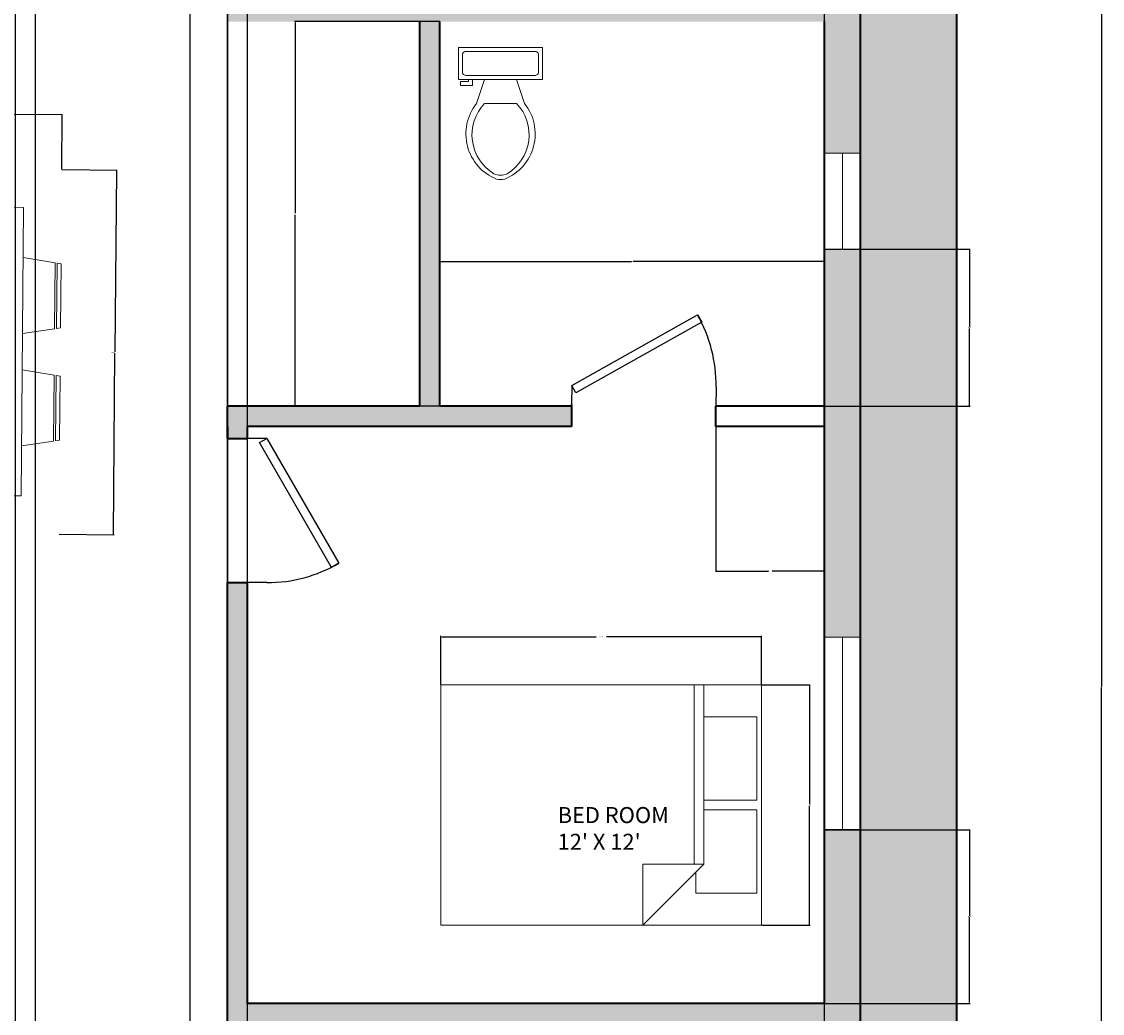
# Model space of a CAD drawing. Units: inches. Extents: x -7 to 546, y -27 to 766.
# Tile 8 of 9: x 276 to 546, y 276 to 524. Entities that reach past the tile are written whole.
import ezdxf

# ---------------------------------------------------------------- set-up
doc = ezdxf.new("R2010")
doc.units = ezdxf.units.IN
doc.header["$MEASUREMENT"] = 0
for name, color, linetype, lineweight in [('A-ANNO-DIMS', 2, 'Continuous', 18), ('A-AREA-IDEN', 7, 'Continuous', 18), ('A-FLOR-FIXT', 9, 'Continuous', 18), ('A-WALL', 7, 'Continuous', 35), ('C-PROP', 7, 'Continuous', 35), ('doors', 40, 'Continuous', 25), ('furniture', 220, 'Continuous', 18), ('window', 30, 'Continuous', 20)]:
    doc.layers.add(name, color=color, linetype=linetype, lineweight=lineweight)
doc.layers.add('A-WALL-PATT', color=251, linetype='Continuous', lineweight=13, true_color=0x636466)
doc.layers.add('L-PLNT-PATT', color=85, linetype='Continuous', lineweight=13, true_color=0x58ba48)
doc.styles.get("Standard").update_dxf_attribs({"font": 'arial.ttf'})
doc.dimstyles.get("Standard").update_dxf_attribs({"dimtxt": 0.18, "dimasz": 0.18, "dimexe": 0.18, "dimexo": 0.0625, "dimgap": 0.09, "dimtad": 0, "dimtih": 1, "dimtoh": 1, "dimdec": 4, "dimzin": 0, "dimdsep": 46, "dimtxsty": 'Standard', "dimcen": 0.09, "dimadec": 0, "dimazin": 0, "dimtfac": 1, "dimtdec": 4, "dimtofl": 0, "dimtmove": 0, "dimatfit": 3, "dimfxl": 1, "dimtolj": 1, "dimtzin": 0, "dimarcsym": 0})

# ---------------------------------------------------------------- blocks, each defined once
blk = doc.blocks.new('*U10')
for p, q in [((0, 0), (0, -100)), ((750, 0), (750, -100))]:
    blk.add_line(p, q)
blk.add_lwpolyline([(0, 0), (649.5, 375), (671.4, 337.1), (21.9, -37.9)], close=True)
blk.add_arc((0, 0), 750, 0, 30)
blk = doc.blocks.new('Dining Set - 36 x 72 in.')
for p, q in [((-22, 27.5), (-22.1562, 26.50042)), ((-22, 27.5), (-6, 27.5)), ((-5.8437, 26.49966), (-6, 27.5)), ((6, 27.5), (5.8438, 26.50042)), ((6, 27.5), (22, 27.5)), ((22.1563, 26.49966), (22, 27.5)), ((-22.2343, 26.00059), (-23.4847, 17.99762)), ((-22.2304, 26), (-5.7608, 26)), ((-5.8416, 26.5), (-22.1534, 26.5)), ((-4.5152, 17.99762), (-5.7655, 25.99926)), ((5.7657, 26.00059), (4.5153, 17.99762)), ((5.7696, 26), (22.2392, 26)), ((22.1584, 26.5), (5.8466, 26.5)), ((23.4848, 17.99762), (22.2345, 25.99926)), ((36, 18), (-36, 18)), ((-36, 18), (-36, -18)), ((36, -18), (36, 18)), ((-45.5, 8), (-44.5004, 8.15617)), ((-44.5, -8.15843), (-44.5, 8.15338)), ((-44.0006, 8.23428), (-35.9976, 9.48474)), ((-44, 8.23041), (-44, -8.23915)), ((44.0006, 8.23428), (35.9976, 9.48474)), ((44, 8.23041), (44, -8.23915)), ((44.5, -8.15843), (44.5, 8.15338)), ((45.5, 8), (44.5005, 8.15617)), ((-45.5, 8), (-45.5, -8)), ((45.5, 8), (45.5, -8)), ((-44.4997, -8.15631), (-45.5, -8)), ((44.4997, -8.15631), (45.5, -8)), ((-35.9976, -9.48476), (-43.9993, -8.2345)), ((35.9976, -9.48476), (43.9993, -8.2345)), ((-36, -18), (36, -18)), ((-22.2343, -26.0006), (-23.4847, -17.99762)), ((-4.5152, -17.99762), (-5.7655, -25.99928)), ((5.7657, -26.0006), (4.5153, -17.99762)), ((23.4848, -17.99762), (22.2345, -25.99928)), ((-22.2304, -26), (-5.7608, -26)), ((-22, -27.5), (-22.1562, -26.50044)), ((-5.8416, -26.5), (-22.1534, -26.5)), ((-5.8437, -26.49967), (-6, -27.5)), ((5.7696, -26), (22.2392, -26)), ((6, -27.5), (5.8438, -26.50044)), ((22.1584, -26.5), (5.8466, -26.5)), ((22.1563, -26.49967), (22, -27.5)), ((-22, -27.5), (-6, -27.5)), ((6, -27.5), (22, -27.5))]:
    blk.add_line(p, q)
for points in [[(-36, 15), (-31.1772, 14.97754), (-26.8079, 14.91406), (-22.8538, 14.81543), (-19.276, 14.6875), (-16.0362, 14.53613), (-13.0957, 14.36718), (-10.4159, 14.18652), (-7.9583, 14), (-5.6904, 13.81315), (-3.6035, 13.63021), (-1.6954, 13.45508), (0.0365, 13.29166), (1.5945, 13.14388), (2.9811, 13.01562), (4.1988, 12.9108), (5.25, 12.83333), (6.1393, 12.78613), (6.8802, 12.76823), (7.4883, 12.77767), (7.9792, 12.8125), (8.3685, 12.87077), (8.6719, 12.95052), (8.9049, 13.0498), (9.0833, 13.16666), (9.2205, 13.29899), (9.3216, 13.44401), (9.3895, 13.59879), (9.4271, 13.76041), (9.4373, 13.92594), (9.4232, 14.09245), (9.3875, 14.257), (9.3333, 14.41666), (9.2638, 14.56917), (9.1836, 14.71484), (9.0975, 14.85465), (9.0104, 14.98958), (8.9272, 15.1206), (8.8529, 15.2487), (8.7922, 15.37483), (8.75, 15.5), (8.7305, 15.62467), (8.7344, 15.74739), (8.7617, 15.86621), (8.8125, 15.97916), (8.8867, 16.08431), (8.9844, 16.17968), (9.1055, 16.26334), (9.25, 16.33333), (9.4189, 16.38802), (9.6172, 16.42708), (9.8506, 16.45052), (10.125, 16.45833), (10.4463, 16.45052), (10.8203, 16.42708), (11.2529, 16.38802), (11.75, 16.33333), (12.3184, 16.26318), (12.9694, 16.17838), (13.7151, 16.07991), (14.5677, 15.96875), (15.5395, 15.84586), (16.6426, 15.71224), (17.8893, 15.56884), (19.2917, 15.41666), (20.859, 15.25667), (22.5879, 15.08984), (24.4721, 14.91715), (26.5052, 14.73958), (28.6809, 14.5581), (30.9929, 14.3737), (33.4347, 14.18733), (36, 14)], [(-36, 10), (-28.9766, 10.14274), (-23.1725, 10.20442), (-18.4241, 10.19775), (-14.5677, 10.13541), (-11.4399, 10.03011), (-8.877, 9.89453), (-6.7154, 9.74137), (-4.7917, 9.58333), (-2.9698, 9.43082), (-1.2246, 9.28515), (0.4415, 9.14534), (2.026, 9.01041), (3.5266, 8.87939), (4.9408, 8.7513), (6.266, 8.62516), (7.5, 8.5), (8.6411, 8.37549), (9.6914, 8.2539), (10.6538, 8.13818), (11.5312, 8.03125), (12.3267, 7.93603), (13.043, 7.85547), (13.6831, 7.79248), (14.25, 7.75), (14.7471, 7.7303), (15.1797, 7.73307), (15.5537, 7.75732), (15.875, 7.80208), (16.1494, 7.86637), (16.3828, 7.94922), (16.5811, 8.04964), (16.75, 8.16666), (16.8944, 8.29915), (17.0143, 8.44531), (17.1089, 8.60319), (17.1771, 8.77083), (17.218, 8.94629), (17.2305, 9.1276), (17.2137, 9.31282), (17.1667, 9.5), (17.0895, 9.6875), (16.987, 9.875), (16.8649, 10.0625), (16.7292, 10.25), (16.5856, 10.4375), (16.4401, 10.625), (16.2985, 10.8125), (16.1667, 11), (16.05, 11.18733), (15.9518, 11.3737), (15.8752, 11.5581), (15.8229, 11.73958), (15.798, 11.91715), (15.8034, 12.08984), (15.842, 12.25667), (15.9167, 12.41666), (16.0295, 12.56836), (16.1784, 12.70833), (16.3605, 12.83268), (16.5729, 12.9375), (16.8127, 13.01888), (17.0768, 13.07291), (17.3625, 13.0957), (17.6667, 13.08333), (17.9894, 13.03312), (18.3418, 12.94726), (18.7382, 12.82918), (19.1927, 12.68229), (19.7195, 12.51001), (20.3327, 12.31575), (21.0465, 12.10294), (21.875, 11.875), (22.8357, 11.63354), (23.959, 11.37304), (25.2786, 11.08618), (26.8282, 10.76562), (28.6414, 10.40405), (30.752, 9.99414), (33.1936, 9.52856), (36, 9)], [(-36, 5.5), (-30.7157, 5.3348), (-26.069, 5.20963), (-21.9946, 5.11767), (-18.4271, 5.05208), (-15.3009, 5.00602), (-12.5508, 4.97265), (-10.1112, 4.94515), (-7.9167, 4.91666), (-5.909, 4.88167), (-4.0586, 4.83984), (-2.3429, 4.79215), (-0.7396, 4.73958), (0.7739, 4.6831), (2.22, 4.6237), (3.6213, 4.56233), (5, 4.5), (6.373, 4.43782), (7.7344, 4.3776), (9.0723, 4.32129), (10.375, 4.27083), (11.6309, 4.22819), (12.8281, 4.19531), (13.9551, 4.17415), (15, 4.16666), (15.954, 4.17448), (16.819, 4.19791), (17.6001, 4.23698), (18.3021, 4.29166), (18.9299, 4.36198), (19.4883, 4.44791), (19.9823, 4.54948), (20.4167, 4.66666), (20.7969, 4.79899), (21.1302, 4.94401), (21.4245, 5.09879), (21.6875, 5.26041), (21.9271, 5.42594), (22.1511, 5.59245), (22.3672, 5.757), (22.5834, 5.91666), (22.8065, 6.06868), (23.0404, 6.21093), (23.2879, 6.34147), (23.5521, 6.45833), (23.8358, 6.55957), (24.142, 6.64323), (24.4735, 6.70735), (24.8334, 6.75), (25.2235, 6.76969), (25.642, 6.76692), (26.0858, 6.74267), (26.5521, 6.69791), (27.0379, 6.63362), (27.5404, 6.55078), (28.0565, 6.45036), (28.5834, 6.33333), (29.1242, 6.19987), (29.7071, 6.04687), (30.3661, 5.87044), (31.1354, 5.66666), (32.0493, 5.43164), (33.142, 5.16146), (34.4475, 4.85221), (36, 4.5)], [(-36, -1), (-30.7915, -0.6591), (-26.0195, -0.38216), (-21.6519, -0.16284), (-17.6563, 0.00521), (-14.0005, 0.12833), (-10.6523, 0.21289), (-7.5796, 0.26522), (-4.75, 0.29166), (-2.134, 0.29793), (0.2878, 0.28711), (2.5317, 0.26163), (4.6146, 0.22396), (6.5529, 0.17651), (8.3633, 0.12174), (10.0623, 0.06209), (11.6667, 0), (13.1899, -0.06201), (14.6341, -0.1211), (15.9982, -0.17432), (17.2813, -0.21875), (18.4823, -0.25147), (19.6003, -0.26953), (20.6343, -0.27002), (21.5834, -0.25), (22.4481, -0.20768), (23.2357, -0.14584), (23.9549, -0.06836), (24.6146, 0.02083), (25.2235, 0.11784), (25.7904, 0.21875), (26.3241, 0.31966), (26.8334, 0.41666), (27.3265, 0.50618), (27.8099, 0.58593), (28.2894, 0.65397), (28.7709, 0.70833), (29.2601, 0.74707), (29.763, 0.76823), (30.2855, 0.76985), (30.8334, 0.75), (31.4088, 0.70784), (31.9994, 0.64713), (32.589, 0.57275), (33.1615, 0.48958), (33.7008, 0.4025), (34.1908, 0.3164), (34.6153, 0.23616), (34.9584, 0.16666), (35.2099, 0.11165), (35.3848, 0.07031), (35.504, 0.04069), (35.5886, 0.02083), (35.6594, 0.00879), (35.7377, 0.0026), (35.8442, 0.00032), (36, 0)], [(-36, -6.5), (-27.1843, -6.31267), (-20.084, -6.1263), (-14.469, -5.9419), (-10.1094, -5.76042), (-6.7752, -5.58285), (-4.2363, -5.41016), (-2.2629, -5.24333), (-0.625, -5.08334), (0.8708, -4.93099), (2.2715, -4.78646), (3.5872, -4.64974), (4.8281, -4.52084), (6.0046, -4.39974), (7.127, -4.28646), (8.2053, -4.18099), (9.25, -4.08334), (10.2705, -3.99382), (11.2734, -3.91407), (12.2647, -3.84603), (13.25, -3.79167), (14.2354, -3.75293), (15.2266, -3.73177), (16.2295, -3.73015), (17.25, -3.75), (18.2912, -3.79248), (19.3451, -3.85547), (20.4009, -3.93604), (21.4479, -4.03125), (22.4754, -4.13819), (23.4727, -4.25391), (24.4289, -4.37549), (25.3334, -4.5), (26.1785, -4.62492), (26.9694, -4.74935), (27.7145, -4.87281), (28.4219, -4.99479), (29.1, -5.11483), (29.7572, -5.23242), (30.4016, -5.34709), (31.0417, -5.45834), (31.6837, -5.56437), (32.3262, -5.65821), (32.9658, -5.73153), (33.599, -5.77604), (34.2224, -5.78345), (34.8327, -5.74545), (35.4264, -5.65373), (36, -5.5)], [(-36, -10), (-26.4022, -9.81299), (-18.4675, -9.62891), (-11.9839, -9.45069), (-6.7396, -9.28125), (-2.5226, -9.12354), (0.8789, -8.98047), (3.6769, -8.85498), (6.0833, -8.75), (8.2767, -8.66765), (10.3021, -8.60677), (12.1712, -8.56543), (13.8958, -8.54167), (15.4876, -8.53353), (16.9583, -8.53907), (18.3197, -8.55632), (19.5834, -8.58334), (20.7616, -8.61841), (21.8685, -8.66081), (22.9188, -8.71004), (23.9271, -8.76563), (24.9081, -8.82707), (25.8763, -8.89388), (26.8465, -8.96558), (27.8334, -9.04167), (28.8474, -9.12118), (29.8828, -9.20117), (30.93, -9.27824), (31.9792, -9.34896), (33.0205, -9.40991), (34.0443, -9.45768), (35.0407, -9.48885), (36, -9.5)], [(-36, -14.5), (-30.0881, -14.33513), (-25.0332, -14.21224), (-20.7312, -14.12647), (-17.0781, -14.07292), (-13.97, -14.04671), (-11.3027, -14.04297), (-8.9724, -14.05681), (-6.875, -14.08334), (-4.9224, -14.11833), (-3.0905, -14.16016), (-1.3709, -14.20785), (0.2448, -14.26042), (1.7647, -14.3169), (3.1973, -14.3763), (4.5507, -14.43767), (5.8333, -14.5), (7.0554, -14.5621), (8.235, -14.62175), (9.3922, -14.67652), (10.5469, -14.72396), (11.7192, -14.76164), (12.929, -14.78711), (14.1965, -14.79794), (15.5417, -14.79167), (16.9933, -14.76424), (18.6152, -14.70508), (20.4804, -14.60197), (22.6615, -14.44271), (25.2312, -14.21509), (28.2624, -13.9069), (31.8277, -13.50594), (36, -13)]]:
    blk.add_lwpolyline(points)
blk = doc.blocks.new('Bed - Queen')
for p, q in [((0, -80.00003), (0, 0)), ((0, 0), (59.99999, 0)), ((59.99999, 0), (59.99999, -80.00003)), ((7.99999, -1.2), (28.79998, -1.2)), ((7.99999, -14.4), (7.99999, -1.2)), ((28.79998, -1.2), (28.79998, -14.4)), ((31.19999, -1.2), (51.99999, -1.2)), ((31.19999, -14.4), (31.19999, -1.2)), ((51.99999, -1.2), (51.99999, -16.4)), ((0, -14.4), (44.8, -14.4)), ((59.99999, -29.6), (44.8, -14.4)), ((44.8, -14.4), (44.8, -29.6)), ((44.8, -16.8), (0, -16.8)), ((51.99999, -16.4), (46.79936, -16.4)), ((44.8, -29.6), (59.99999, -29.6)), ((59.99999, -80.00003), (0, -80.00003))]:
    blk.add_line(p, q)
blk = doc.blocks.new('Toilet - top')
for p, q in [((9.5, -6), (9.5, -2)), ((-8, -8.5), (-8, -8)), ((-7, -8), (-7, -9.5)), ((-4, -8), (-6, -14)), ((4, -8), (6, -14)), ((-10, -8.5), (-8, -8.5)), ((-10, -9.5), (-10, -8.5)), ((-7, -9.5), (-10, -9.5)), ((4, -14), (-4, -14))]:
    blk.add_line(p, q)
blk.add_lwpolyline([(10.5, -8), (10.5, 0), (-10.5, 0), (-10.5, -8)], close=True)
for points in [[(-9.5, -2), (-9.5, -6)], [(8.5, -1), (-8.5, -1)], [(-8.5, -7), (8.5, -7)]]:
    blk.add_lwpolyline(points)
for centre, radius, start, end in [((-8.62, -1.88), 0.884, 81.8699, 188.1301), ((8.62, -1.88), 0.884, 351.8699, 98.1301), ((-8.62, -6.12), 0.884, 171.8699, 278.1301), ((8.62, -6.12), 0.884, 261.8699, 8.1301), ((3.52, -21.58), 12.17, 141.4691, 247.9714), ((4.2, -21.82), 11.33, 136.3677, 238.9468), ((-3.52, -21.58), 12.17, 292.0284, 38.5307), ((-4.2, -21.82), 11.33, 301.053, 43.6321), ((0, -27.88), 4, 245.7318, 294.2682), ((0, -29), 4, 254.8605, 285.1395)]:
    blk.add_arc(centre, radius, start, end)
blk = doc.blocks.new('WIN-48IN')
for p, q in [((0, 9), (0, 0)), ((48, 9), (0, 9)), ((0, 9), (0, 4.5)), ((48, 0), (48, 9)), ((0, 4.5), (48, 4.5)), ((0, 0), (48, 0))]:
    blk.add_line(p, q)
blk = doc.blocks.new('WIN-24IN')
for p, q in [((0, 9), (0, 0)), ((24, 9), (0, 9)), ((0, 9), (0, 4.5)), ((24, 0), (24, 9)), ((0, 4.5), (24, 4.5)), ((0, 0), (24, 0))]:
    blk.add_line(p, q)
blk = doc.blocks.new('*D18')
at = {"layer": 'A-ANNO-DIMS', "color": 0, "lineweight": -2, "transparency": 16777216}
for p, q in [((380.49, 358.31), (380.49, 370.43)), ((380.67, 370.25), (419.19, 370.25)), ((460.31, 370.25), (421.79, 370.25)), ((460.49, 358.31), (460.49, 370.43))]:
    blk.add_line(p, q, dxfattribs=at)
at = {"layer": 'A-ANNO-DIMS', "color": 0, "transparency": 16777216}
for points in [[(380.67, 370.28), (380.67, 370.22), (380.49, 370.25)], [(460.31, 370.28), (460.31, 370.22), (460.49, 370.25)]]:
    blk.add_solid(points, dxfattribs=at)
at = {"layer": 'Defpoints', "color": 0, "transparency": 16777216}
for p in [(460.49, 370.25), (380.49, 358.25), (460.49, 358.25)]:
    blk.add_point(p, dxfattribs=at)
at = {"layer": 'A-ANNO-DIMS', "color": 0, "transparency": 16777216, "insert": (420.49, 370.25), "char_height": 0.18, "attachment_point": 5}
blk.add_mtext('\\A1;QUEEN BED 80 TYP.', dxfattribs=at)
blk = doc.blocks.new('*D19')
at = {"layer": 'A-ANNO-DIMS', "color": 0, "lineweight": -2, "transparency": 16777216}
for p, q in [((460.55, 358.25), (472.67, 358.25)), ((472.49, 358.07), (472.49, 328.43)), ((472.49, 298.43), (472.49, 328.07)), ((460.55, 298.25), (472.67, 298.25))]:
    blk.add_line(p, q, dxfattribs=at)
at = {"layer": 'A-ANNO-DIMS', "color": 0, "transparency": 16777216}
for points in [[(472.46, 358.07), (472.52, 358.07), (472.49, 358.25)], [(472.46, 298.43), (472.52, 298.43), (472.49, 298.25)]]:
    blk.add_solid(points, dxfattribs=at)
at = {"layer": 'Defpoints', "color": 0, "transparency": 16777216}
for p in [(460.49, 358.25), (460.49, 298.25), (472.49, 298.25)]:
    blk.add_point(p, dxfattribs=at)
at = {"layer": 'A-ANNO-DIMS', "color": 0, "transparency": 16777216, "insert": (472.49, 328.25), "char_height": 0.18, "attachment_point": 5}
blk.add_mtext('\\A1;60 TYP.', dxfattribs=at)
blk = doc.blocks.new('*D24')
at = {"layer": 'A-ANNO-DIMS', "color": 0, "lineweight": -2, "transparency": 16777216}
for p, q in [((285.93, 486.8), (299.7, 486.69)), ((299.52, 486.51), (299.14, 441.37)), ((298.76, 395.87), (299.14, 441.01)), ((285.18, 395.8), (298.94, 395.69))]:
    blk.add_line(p, q, dxfattribs=at)
at = {"layer": 'A-ANNO-DIMS', "color": 0, "transparency": 16777216}
for points in [[(299.49, 486.51), (299.55, 486.51), (299.52, 486.69)], [(298.73, 395.87), (298.79, 395.87), (298.76, 395.69)]]:
    blk.add_solid(points, dxfattribs=at)
at = {"layer": 'Defpoints', "color": 0, "transparency": 16777216}
for p in [(285.87, 486.8), (299.52, 486.69), (285.11, 395.81)]:
    blk.add_point(p, dxfattribs=at)
at = {"layer": 'A-ANNO-DIMS', "color": 0, "transparency": 16777216, "insert": (299.14, 441.19), "char_height": 0.18, "attachment_point": 5}
blk.add_mtext('\\A1;DINING SET 91', dxfattribs=at)
blk = doc.blocks.new('*D25')
at = {"layer": 'A-ANNO-DIMS', "color": 0, "lineweight": -2, "transparency": 16777216}
for p, q in [((230.87, 487.32), (230.98, 501.09)), ((231.16, 500.91), (258.26, 500.68)), ((285.8, 500.45), (258.7, 500.68)), ((285.87, 486.86), (285.98, 500.63))]:
    blk.add_line(p, q, dxfattribs=at)
at = {"layer": 'A-ANNO-DIMS', "color": 0, "transparency": 16777216}
for points in [[(231.16, 500.94), (231.16, 500.88), (230.98, 500.91)], [(285.8, 500.48), (285.8, 500.42), (285.98, 500.45)]]:
    blk.add_solid(points, dxfattribs=at)
at = {"layer": 'Defpoints', "color": 0, "transparency": 16777216}
for p in [(230.98, 500.91), (230.87, 487.26), (285.87, 486.8)]:
    blk.add_point(p, dxfattribs=at)
at = {"layer": 'A-ANNO-DIMS', "color": 0, "transparency": 16777216, "insert": (258.48, 500.68), "char_height": 0.18, "attachment_point": 5}
blk.add_mtext('\\A1;55', dxfattribs=at)
blk = doc.blocks.new('*D33')
at = {"layer": 'A-ANNO-DIMS', "color": 0, "lineweight": -2, "transparency": 16777216}
for p, q in [((485.29, 705.74), (545.54, 705.74)), ((545.36, 705.56), (545.36, 357.93)), ((545.36, 9.92), (545.36, 357.56)), ((461.29, 9.74), (545.54, 9.74))]:
    blk.add_line(p, q, dxfattribs=at)
at = {"layer": 'A-ANNO-DIMS', "color": 0, "transparency": 16777216}
for points in [[(545.33, 705.56), (545.39, 705.56), (545.36, 705.74)], [(545.33, 9.92), (545.39, 9.92), (545.36, 9.74)]]:
    blk.add_solid(points, dxfattribs=at)
at = {"layer": 'Defpoints', "color": 0, "transparency": 16777216}
for p in [(485.23, 705.74), (461.23, 9.74), (545.36, 9.74)]:
    blk.add_point(p, dxfattribs=at)
at = {"layer": 'A-ANNO-DIMS', "color": 0, "transparency": 16777216, "insert": (545.36, 357.74), "char_height": 0.18, "attachment_point": 5}
blk.add_mtext('\\A1;696', dxfattribs=at)
blk = doc.blocks.new('*D41')
at = {"layer": 'A-ANNO-DIMS', "color": 0, "lineweight": -2, "transparency": 16777216}
for p, q in [((274.23, 600.68), (274.23, -26.56)), ((279.23, 600.68), (279.23, -26.56)), ((274.41, -26.38), (276.58, -26.38)), ((279.05, -26.38), (276.88, -26.38))]:
    blk.add_line(p, q, dxfattribs=at)
at = {"layer": 'A-ANNO-DIMS', "color": 0, "transparency": 16777216}
for points in [[(274.41, -26.35), (274.41, -26.41), (274.23, -26.38)], [(279.05, -26.35), (279.05, -26.41), (279.23, -26.38)]]:
    blk.add_solid(points, dxfattribs=at)
at = {"layer": 'Defpoints', "color": 0, "transparency": 16777216}
for p in [(274.23, 600.74), (279.23, 600.74), (279.23, -26.38)]:
    blk.add_point(p, dxfattribs=at)
at = {"layer": 'A-ANNO-DIMS', "color": 0, "transparency": 16777216, "insert": (276.73, -26.38), "char_height": 0.18, "attachment_point": 5}
blk.add_mtext('\\A1;5', dxfattribs=at)
blk = doc.blocks.new('*D43')
at = {"layer": 'A-ANNO-DIMS', "color": 0, "lineweight": -2, "transparency": 16777216}
for p, q in [((317.84, 696.68), (317.84, -26.56)), ((327.23, 696.68), (327.23, -26.56)), ((318.02, -26.38), (322.21, -26.38)), ((327.05, -26.38), (322.86, -26.38))]:
    blk.add_line(p, q, dxfattribs=at)
at = {"layer": 'A-ANNO-DIMS', "color": 0, "transparency": 16777216}
for points in [[(318.02, -26.35), (318.02, -26.41), (317.84, -26.38)], [(327.05, -26.35), (327.05, -26.41), (327.23, -26.38)]]:
    blk.add_solid(points, dxfattribs=at)
at = {"layer": 'Defpoints', "color": 0, "transparency": 16777216}
for p in [(317.84, 696.74), (327.23, 696.74), (327.23, -26.38)]:
    blk.add_point(p, dxfattribs=at)
at = {"layer": 'A-ANNO-DIMS', "color": 0, "transparency": 16777216, "insert": (322.54, -26.38), "char_height": 0.18, "attachment_point": 5}
blk.add_mtext('\\A1;9.39', dxfattribs=at)
blk = doc.blocks.new('*D46')
at = {"layer": 'A-ANNO-DIMS', "color": 0, "lineweight": -2, "transparency": 16777216}
for p, q in [((380.23, 427.81), (380.23, 464.05)), ((476.23, 427.81), (476.23, 464.05)), ((380.41, 463.87), (428.01, 463.87)), ((476.05, 463.87), (428.45, 463.87))]:
    blk.add_line(p, q, dxfattribs=at)
at = {"layer": 'A-ANNO-DIMS', "color": 0, "transparency": 16777216}
for points in [[(380.41, 463.9), (380.41, 463.84), (380.23, 463.87)], [(476.05, 463.9), (476.05, 463.84), (476.23, 463.87)]]:
    blk.add_solid(points, dxfattribs=at)
at = {"layer": 'Defpoints', "color": 0, "transparency": 16777216}
for p in [(476.23, 463.87), (380.23, 427.74), (476.23, 427.74)]:
    blk.add_point(p, dxfattribs=at)
at = {"layer": 'A-ANNO-DIMS', "color": 0, "transparency": 16777216, "insert": (428.23, 463.87), "char_height": 0.18, "attachment_point": 5}
blk.add_mtext('\\A1;96', dxfattribs=at)
blk = doc.blocks.new('*D47')
at = {"layer": 'A-ANNO-DIMS', "color": 0, "lineweight": -2, "transparency": 16777216}
for p, q in [((380.17, 523.74), (343.93, 523.74)), ((344.11, 523.56), (344.11, 475.93)), ((344.11, 427.92), (344.11, 475.56)), ((380.17, 427.74), (343.93, 427.74))]:
    blk.add_line(p, q, dxfattribs=at)
at = {"layer": 'A-ANNO-DIMS', "color": 0, "transparency": 16777216}
for points in [[(344.08, 523.56), (344.14, 523.56), (344.11, 523.74)], [(344.08, 427.92), (344.14, 427.92), (344.11, 427.74)]]:
    blk.add_solid(points, dxfattribs=at)
at = {"layer": 'Defpoints', "color": 0, "transparency": 16777216}
for p in [(344.11, 523.74), (380.23, 523.74), (380.23, 427.74)]:
    blk.add_point(p, dxfattribs=at)
at = {"layer": 'A-ANNO-DIMS', "color": 0, "transparency": 16777216, "insert": (344.11, 475.74), "char_height": 0.18, "attachment_point": 5}
blk.add_mtext('\\A1;96', dxfattribs=at)
blk = doc.blocks.new('*D57')
at = {"layer": 'A-ANNO-DIMS', "color": 0, "lineweight": -2, "transparency": 16777216}
for p, q in [((332.23, 273.81), (332.23, 766.05)), ((476.23, 273.81), (476.23, 766.05)), ((332.41, 765.87), (403.95, 765.87)), ((476.05, 765.87), (404.51, 765.87))]:
    blk.add_line(p, q, dxfattribs=at)
at = {"layer": 'A-ANNO-DIMS', "color": 0, "transparency": 16777216}
for points in [[(332.41, 765.9), (332.41, 765.84), (332.23, 765.87)], [(476.05, 765.9), (476.05, 765.84), (476.23, 765.87)]]:
    blk.add_solid(points, dxfattribs=at)
at = {"layer": 'Defpoints', "color": 0, "transparency": 16777216}
for p in [(476.23, 765.87), (332.23, 273.74), (476.23, 273.74)]:
    blk.add_point(p, dxfattribs=at)
at = {"layer": 'A-ANNO-DIMS', "color": 0, "transparency": 16777216, "insert": (404.23, 765.87), "char_height": 0.18, "attachment_point": 5}
blk.add_mtext('\\A1;144', dxfattribs=at)
blk = doc.blocks.new('*D76')
at = {"layer": 'A-ANNO-DIMS', "color": 0, "lineweight": -2, "transparency": 16777216}
for p, q in [((476.29, 322.09), (512.54, 322.09)), ((512.36, 321.91), (512.36, 300.6)), ((512.36, 278.92), (512.36, 300.24)), ((476.29, 278.74), (512.54, 278.74))]:
    blk.add_line(p, q, dxfattribs=at)
at = {"layer": 'A-ANNO-DIMS', "color": 0, "transparency": 16777216}
for points in [[(512.33, 321.91), (512.39, 321.91), (512.36, 322.09)], [(512.33, 278.92), (512.39, 278.92), (512.36, 278.74)]]:
    blk.add_solid(points, dxfattribs=at)
at = {"layer": 'Defpoints', "color": 0, "transparency": 16777216}
for p in [(476.23, 322.09), (476.23, 278.74), (512.36, 278.74)]:
    blk.add_point(p, dxfattribs=at)
at = {"layer": 'A-ANNO-DIMS', "color": 0, "transparency": 16777216, "insert": (512.36, 300.42), "char_height": 0.18, "attachment_point": 5}
blk.add_mtext('\\A1;43.35', dxfattribs=at)
blk = doc.blocks.new('*D77')
at = {"layer": 'A-ANNO-DIMS', "color": 0, "lineweight": -2, "transparency": 16777216}
for p, q in [((476.29, 466.93), (512.54, 466.93)), ((512.36, 466.75), (512.36, 447.52)), ((512.36, 427.92), (512.36, 447.16)), ((476.29, 427.74), (512.54, 427.74))]:
    blk.add_line(p, q, dxfattribs=at)
at = {"layer": 'A-ANNO-DIMS', "color": 0, "transparency": 16777216}
for points in [[(512.33, 466.75), (512.39, 466.75), (512.36, 466.93)], [(512.33, 427.92), (512.39, 427.92), (512.36, 427.74)]]:
    blk.add_solid(points, dxfattribs=at)
at = {"layer": 'Defpoints', "color": 0, "transparency": 16777216}
for p in [(476.23, 466.93), (476.23, 427.74), (512.36, 427.74)]:
    blk.add_point(p, dxfattribs=at)
at = {"layer": 'A-ANNO-DIMS', "color": 0, "transparency": 16777216, "insert": (512.36, 447.34), "char_height": 0.18, "attachment_point": 5}
blk.add_mtext('\\A1;39.19', dxfattribs=at)
blk = doc.blocks.new('*D78')
at = {"layer": 'A-ANNO-DIMS', "color": 0, "lineweight": -2, "transparency": 16777216}
for p, q in [((449.09, 422.68), (449.09, 386.44)), ((476.23, 422.68), (476.23, 386.44)), ((449.27, 386.62), (462.2, 386.62)), ((476.05, 386.62), (463.13, 386.62))]:
    blk.add_line(p, q, dxfattribs=at)
at = {"layer": 'A-ANNO-DIMS', "color": 0, "transparency": 16777216}
for points in [[(449.27, 386.65), (449.27, 386.59), (449.09, 386.62)], [(476.05, 386.65), (476.05, 386.59), (476.23, 386.62)]]:
    blk.add_solid(points, dxfattribs=at)
at = {"layer": 'Defpoints', "color": 0, "transparency": 16777216}
for p in [(449.09, 422.74), (476.23, 422.74), (449.09, 386.62)]:
    blk.add_point(p, dxfattribs=at)
at = {"layer": 'A-ANNO-DIMS', "color": 0, "transparency": 16777216, "insert": (462.66, 386.62), "char_height": 0.18, "attachment_point": 5}
blk.add_mtext('\\A1;27.143', dxfattribs=at)
blk = doc.blocks.new('*D81')
at = {"layer": 'A-ANNO-DIMS', "color": 0, "lineweight": -2, "transparency": 16777216}
for p, q in [((62.23, 240.81), (62.23, 766.05)), ((327.23, 234.81), (327.23, 766.05)), ((62.41, 765.87), (194.44, 765.87)), ((327.05, 765.87), (195.02, 765.87))]:
    blk.add_line(p, q, dxfattribs=at)
at = {"layer": 'A-ANNO-DIMS', "color": 0, "transparency": 16777216}
for points in [[(62.41, 765.9), (62.41, 765.84), (62.23, 765.87)], [(327.05, 765.9), (327.05, 765.84), (327.23, 765.87)]]:
    blk.add_solid(points, dxfattribs=at)
at = {"layer": 'Defpoints', "color": 0, "transparency": 16777216}
for p in [(327.23, 765.87), (62.23, 240.74), (327.23, 234.74)]:
    blk.add_point(p, dxfattribs=at)
at = {"layer": 'A-ANNO-DIMS', "color": 0, "transparency": 16777216, "insert": (194.73, 765.87), "char_height": 0.18, "attachment_point": 5}
blk.add_mtext('\\A1;265', dxfattribs=at)

msp = doc.modelspace()

# ---------------------------------------------------------------- hatches: boundary and pattern name
at = {"layer": 'A-WALL-PATT'}
h = msp.add_hatch(color=256, dxfattribs=at)
h.dxf.hatch_style = 1
h.paths.add_polyline_path([(62.2319, 696.744), (86.6896, 696.744), (86.6896, 705.744), (53.2319, 705.744), (53.2319, 627.8642), (57.7271, 627.8642), (62.2319, 627.8642)])
h.paths.add_polyline_path([(229.7414, 705.744), (134.6896, 705.744), (134.6896, 696.744), (206.2319, 696.744), (206.2319, 567.744), (211.2319, 567.744), (211.2319, 595.744), (214.2319, 595.744), (214.2319, 600.744), (211.2319, 600.744), (211.2319, 696.744), (229.7414, 696.744)])
h.paths.add_polyline_path([(293.8423, 705.744), (253.7414, 705.744), (253.7414, 696.744), (274.2319, 696.744), (274.2319, 600.744), (279.2319, 600.744), (279.2319, 696.744), (293.8423, 696.744)])
h.paths.add_polyline_path([(393.9743, 705.744), (317.8423, 705.744), (317.8423, 696.744), (327.2319, 696.744), (327.2319, 651.744), (332.2319, 651.744), (332.2319, 696.744), (393.9743, 696.744)])
h.paths.add_polyline_path([(485.2319, 705.744), (441.9743, 705.744), (441.9743, 696.744), (476.2319, 696.744), (476.2319, 663.6898), (480.7319, 663.6898), (485.2319, 663.6898)])
h.paths.add_polyline_path([(485.2319, 615.6898), (476.2319, 615.6898), (476.2319, 528.744), (332.2319, 528.744), (332.2319, 531.744), (327.2319, 531.744), (327.2319, 523.744), (375.2319, 523.744), (375.2319, 427.744), (327.2319, 427.744), (327.2319, 419.744), (332.2319, 419.744), (332.2319, 422.744), (413.089, 422.744), (413.089, 427.744), (380.2319, 427.744), (380.2319, 523.744), (476.2319, 523.744), (476.2319, 490.9334), (485.2319, 490.9334)])
h.paths.add_polyline_path([(485.2319, 466.9334), (476.2319, 466.9334), (476.2319, 370.0932), (480.7319, 370.0932), (485.2319, 370.0932)])
h.paths.add_polyline_path([(485.2319, 322.0932), (476.2319, 322.0932), (476.2319, 278.744), (332.2319, 278.744), (332.2319, 383.744), (327.2319, 383.744), (327.2319, 273.744), (327.2319, 270.744), (332.2319, 270.744), (332.2319, 273.744), (476.2319, 273.744), (476.2319, 201.0338), (480.7319, 201.0338), (485.2319, 201.0338)])
h.paths.add_polyline_path([(485.2319, 153.0338), (476.2319, 153.0338), (476.2319, 42.744), (461.2319, 42.744), (461.2319, 33.744), (485.2319, 33.744)])
h.paths.add_polyline_path([(332.2319, 234.744), (327.2319, 234.744), (327.2319, 160.744), (315.2319, 160.744), (315.2319, 151.744), (327.2319, 151.744), (327.2319, 33.744), (332.2319, 33.744)])
h.paths.add_polyline_path([(252.2319, 151.744), (258.4464, 151.744), (264.2319, 151.744), (264.2319, 160.744), (252.2319, 160.744), (252.2319, 172.744), (247.2319, 172.744), (247.2319, 91.744), (127.2319, 91.744), (127.2319, 196.744), (122.2319, 196.744), (122.2319, 91.744), (62.2319, 91.744), (62.2319, 126.1124), (53.2319, 126.1124), (53.2319, 9.744), (62.2319, 9.744), (62.2319, 86.744), (247.2319, 86.744), (247.2319, 33.744), (252.2319, 33.744), (252.2319, 53.744)])
h.paths.add_polyline_path([(62.2319, 235.744), (122.2319, 235.744), (122.2319, 232.744), (127.2319, 232.744), (127.2319, 235.744), (247.2319, 235.744), (247.2319, 220.744), (252.2319, 220.744), (252.2319, 240.744), (250.6678, 240.744), (247.2319, 240.744), (62.2319, 240.744), (62.2319, 322.0932), (53.2319, 322.0932), (53.2319, 174.1124), (57.7271, 174.1124), (62.2319, 174.1124)])
at = {"layer": 'L-PLNT-PATT'}
h = msp.add_hatch(color=256, dxfattribs=at)
h.dxf.hatch_style = 1
h.paths.add_polyline_path([(509.2319, 729.744), (29.2319, 729.744), (29.2319, 9.744), (53.2319, 9.744), (53.2319, 705.744), (485.2319, 705.744), (485.2319, 33.744), (461.2319, 33.744), (461.2319, 9.744), (509.2319, 9.744)])

# ---------------------------------------------------------------- linework, layer by layer
at = {"layer": 'A-WALL'}
for p, q in [((375.2319, 427.744), (375.2319, 523.744)), ((380.2319, 427.744), (380.2319, 523.744)), ((476.2319, 278.744), (476.2319, 523.744)), ((327.2319, 419.744), (327.2319, 427.744)), ((375.2319, 427.744), (327.2319, 427.744)), ((413.089, 427.744), (380.2319, 427.744)), ((413.089, 428.1721), (413.089, 422.744)), ((476.2319, 427.744), (449.089, 427.744)), ((449.089, 422.744), (449.089, 427.744)), ((327.2319, 422.744), (327.2319, 419.744)), ((332.2319, 419.744), (332.2319, 422.744)), ((413.089, 422.744), (332.2319, 422.744)), ((476.2319, 422.744), (449.089, 422.744)), ((327.2319, 419.744), (332.2319, 419.744)), ((327.2319, 273.744), (327.2319, 383.744)), ((327.2319, 383.744), (332.2319, 383.744)), ((332.2319, 278.744), (332.2319, 383.744)), ((476.2319, 278.744), (332.2319, 278.744))]:
    msp.add_line(p, q, dxfattribs=at)
msp.add_lwpolyline([(461.2319, 33.744), (485.2319, 33.744), (485.2319, 705.744), (53.2319, 705.744), (53.2319, 9.744)], dxfattribs=at)
at = {"layer": 'C-PROP'}
msp.add_lwpolyline([(29.2319, 9.744), (509.2319, 9.744), (509.2319, 729.744), (29.2319, 729.744)], close=True, dxfattribs=at)

# ---------------------------------------------------------------- block references
at = {"layer": 'A-FLOR-FIXT'}
msp.add_blockref('Toilet - top', (395.3602, 517.3106), dxfattribs=at)
at = {"layer": 'doors'}
for p, xscale, yscale, zscale, rotation in [((413.1461, 432.9721), 0.0480033934064386, 0.0480033934064386, 0.0480033934064386, 359.3187254601357), ((337.0319, 419.744), 0.0479999999999916, 0.0479999999999916, 0.0479999999999916, 269.9999999999971)]:
    msp.add_blockref('*U10', p, dxfattribs=dict(at, xscale=xscale, yscale=yscale, zscale=zscale, rotation=rotation))
at = {"layer": 'furniture'}
for name, p, rotation in [('Dining Set - 36 x 72 in.', (257.9915, 441.5318), 89.5243204840911), ('Bed - Queen', (460.4912, 358.2513), 270)]:
    msp.add_blockref(name, p, dxfattribs=dict(at, rotation=rotation))
at = {"layer": 'window', "rotation": 89.99999999999666}
msp.add_blockref('WIN-24IN', (485.2319, 466.933), dxfattribs=at)
at = {"layer": 'window', "extrusion": (0, 0, -1), "zscale": -1, "rotation": 270.0000000000001}
msp.add_blockref('WIN-48IN', (-485.2319, 370.0928), dxfattribs=at)

# ---------------------------------------------------------------- texts
at = {"layer": 'A-AREA-IDEN', "insert": (409.6063, 327.7332), "char_height": 4, "attachment_point": 1}
msp.add_mtext_dynamic_manual_height_columns("BED ROOM\\P12' X 12'", width=80.777321, gutter_width=1, heights=[0], dxfattribs=at)

# ---------------------------------------------------------------- dimensions: what is measured, and where the dimension line sits
at = {"layer": 'A-ANNO-DIMS'}
for base, p1, p2, override, picture, middle in [((327.2319, 765.869), (62.2319, 240.744), (327.2319, 234.744), {"dimdec": 0, "dimlfac": 1, "dimrnd": 0, "dimzin": 0, "dimdsep": 46, "dimlunit": 2}, '*D81', (194.7319, 765.869)), ((476.2319, 765.869), (332.2319, 273.744), (476.2319, 273.744), {"dimdec": 0, "dimlfac": 1, "dimrnd": 0, "dimzin": 0, "dimdsep": 46, "dimlunit": 2}, '*D57', (404.2319, 765.869)), ((327.2319, -26.381), (317.8423, 696.744), (327.2319, 696.744), {"dimdec": 2, "dimlfac": 1, "dimrnd": 0, "dimzin": 0, "dimdsep": 46, "dimlunit": 2}, '*D43', (322.5371, -26.381)), ((279.2319, -26.381), (274.2319, 600.744), (279.2319, 600.744), {"dimdec": 0, "dimlfac": 1, "dimrnd": 0, "dimzin": 0, "dimdsep": 46, "dimlunit": 2}, '*D41', (276.7319, -26.381)), ((476.2319, 463.869), (380.2319, 427.744), (476.2319, 427.744), {"dimdec": 0, "dimlfac": 1, "dimrnd": 0, "dimzin": 0, "dimdsep": 46, "dimlunit": 2}, '*D46', (428.2319, 463.869))]:
    dim = msp.add_linear_dim(base=base, p1=p1, p2=p2, dimstyle='Standard', override=override, dxfattribs=at)
    dim.commit()
    dim.dimension.update_dxf_attribs({"geometry": picture, "text_midpoint": middle})
for base, p1, p2, angle, override, picture, middle in [((545.3569, 9.744), (485.2319, 705.744), (461.2319, 9.744), 90, {"dimdec": 0, "dimlfac": 1, "dimrnd": 0, "dimzin": 0, "dimdsep": 46, "dimlunit": 2}, '*D33', (545.3569, 357.744)), ((344.1069, 523.744), (380.2319, 427.744), (380.2319, 523.744), 90, {"dimdec": 0, "dimlfac": 1, "dimrnd": 0, "dimzin": 0, "dimdsep": 46, "dimlunit": 2}, '*D47', (344.1069, 475.744)), ((230.9835, 500.908), (285.8683, 486.8019), (230.8702, 487.2585), 179.52432, {"dimdec": 0, "dimlfac": 1, "dimrnd": 0, "dimzin": 0, "dimdsep": 46, "dimlunit": 2}, '*D25', (258.4825, 500.6797)), ((512.3569, 427.744), (476.2319, 466.9334), (476.2319, 427.744), 270, {"dimdec": 2, "dimlfac": 1, "dimrnd": 0, "dimzin": 0, "dimdsep": 46, "dimlunit": 2}, '*D77', (512.3569, 447.3387)), ((449.089, 386.619), (476.2319, 422.744), (449.089, 422.744), 180, {"dimdec": 3, "dimlfac": 1, "dimrnd": 0, "dimzin": 0, "dimdsep": 46, "dimlunit": 2}, '*D78', (462.6605, 386.619)), ((512.3569, 278.744), (476.2319, 322.0932), (476.2319, 278.744), 270, {"dimdec": 2, "dimlfac": 1, "dimrnd": 0, "dimzin": 0, "dimdsep": 46, "dimlunit": 2}, '*D76', (512.3569, 300.4186))]:
    dim = msp.add_linear_dim(base=base, p1=p1, p2=p2, angle=angle, dimstyle='Standard', override=override, dxfattribs=at)
    dim.commit()
    dim.dimension.update_dxf_attribs({"geometry": picture, "text_midpoint": middle})
for base, p1, p2, angle, text, picture, middle in [((299.5178, 486.6886), (285.1128, 395.805), (285.8683, 486.8019), 89.52432, 'DINING SET <>', '*D24', (299.1401, 441.1901)), ((472.4912, 298.2513), (460.4912, 358.2513), (460.4912, 298.2513), 270, '<> TYP.', '*D19', (472.4912, 328.2513))]:
    dim = msp.add_linear_dim(base=base, p1=p1, p2=p2, angle=angle, text=text, dimstyle='Standard', override={"dimdec": 0, "dimlfac": 1, "dimrnd": 0, "dimzin": 0, "dimdsep": 46, "dimlunit": 2}, dxfattribs=at)
    dim.commit()
    dim.dimension.update_dxf_attribs({"geometry": picture, "text_midpoint": middle})
dim = msp.add_linear_dim(base=(460.4912, 370.2513), p1=(380.4912, 358.2513), p2=(460.4912, 358.2513), text='QUEEN BED <> TYP.', dimstyle='Standard', override={"dimdec": 0, "dimlfac": 1, "dimrnd": 0, "dimzin": 0, "dimdsep": 46, "dimlunit": 2}, dxfattribs=at)
dim.commit()
dim.dimension.update_dxf_attribs({"geometry": '*D18', "text_midpoint": (420.4912, 370.2513)})

doc.saveas('drawing.dxf')
